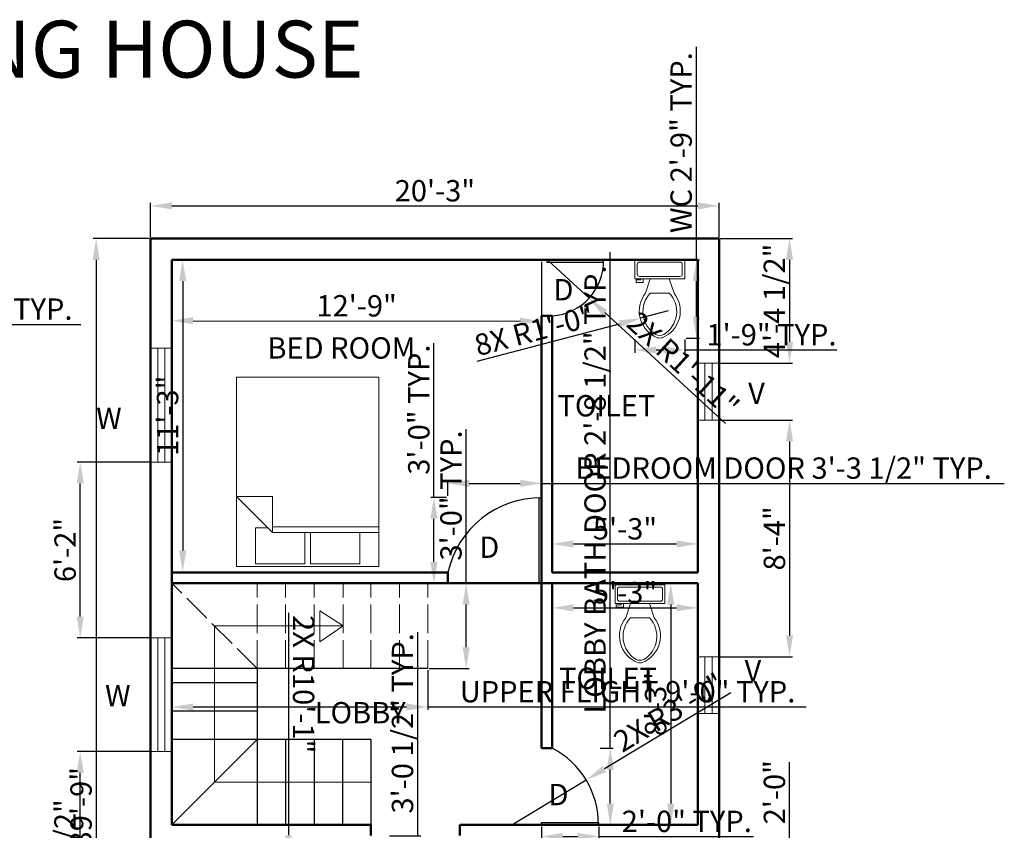
# Model space of a CAD drawing. Units: inches. Extents: x 1802 to 2621, y 1038 to 1686.
# Tile 5 of 5: x 2205 to 2621, y 1344 to 1686. Entities that reach past the tile are written whole.
import ezdxf

# ---------------------------------------------------------------- set-up
doc = ezdxf.new("R2010")
doc.units = ezdxf.units.IN
doc.linetypes.add('ACAD_ISO02W100', pattern=[15, 12, -3])
for name, color, linetype, lineweight in [('A-ANNO-DIMS', 2, 'Continuous', 18), ('A-ANNO-SYMB', 7, 'Continuous', 18), ('A-ANNO-TEXT', 7, 'Continuous', 18), ('A-AREA-IDEN', 7, 'Continuous', 25), ('A-DOOR', 3, 'Continuous', 25), ('A-FLOR-FIXT', 9, 'Continuous', 18), ('A-FLOR-STRS', 7, 'Continuous', 25), ('A-FLOR-STRS-OVHD', 8, 'ACAD_ISO02W100', 18), ('A-FURN', 8, 'Continuous', 18), ('A-GLAZ', 4, 'Continuous', 18), ('A-WALL', 7, 'Continuous', 50)]:
    doc.layers.add(name, color=color, linetype=linetype, lineweight=lineweight)
doc.styles.get("Standard").update_dxf_attribs({"font": 'arial.ttf'})
doc.dimstyles.new('ISO-25', dxfattribs={"dimtxt": 9, "dimasz": 9, "dimexe": 1.25, "dimexo": 0.625, "dimtad": 1, "dimdec": 1, "dimrnd": 9, "dimlunit": 3, "dimtxsty": 'Standard', "dimcen": 2.5, "dimadec": 0, "dimazin": 0, "dimtfac": 1, "dimtdec": 1, "dimtmove": 0, "dimatfit": 3, "dimfxl": 1, "dimarcsym": 0})

# ---------------------------------------------------------------- blocks, each defined once
blk = doc.blocks.new('*D20')
at = {"layer": 'A-ANNO-DIMS', "color": 0, "lineweight": -2, "transparency": 16777216}
for p, q in [((2269.56, 1583.93), (2269.52, 1557.61)), ((2425.56, 1583.74), (2425.52, 1557.42)), ((2278.53, 1558.85), (2416.53, 1558.68))]:
    blk.add_line(p, q, dxfattribs=at)
at = {"layer": 'A-ANNO-DIMS', "color": 0, "transparency": 16777216}
for points in [[(2278.53, 1560.35), (2278.52, 1557.35), (2269.53, 1558.86)], [(2416.53, 1560.18), (2416.52, 1557.18), (2425.53, 1558.67)]]:
    blk.add_solid(points, dxfattribs=at)
at = {"layer": 'Defpoints', "color": 0, "transparency": 16777216}
for p in [(2269.56, 1584.56), (2425.56, 1584.37), (2425.53, 1558.67)]:
    blk.add_point(p, dxfattribs=at)
at = {"layer": 'A-ANNO-DIMS', "color": 0, "transparency": 16777216, "insert": (2347.53, 1563.99), "char_height": 9, "attachment_point": 5, "rotation": 359.9308}
blk.add_mtext('12\'-9"', dxfattribs=at)
blk = doc.blocks.new('*D19')
at = {"layer": 'A-ANNO-DIMS', "color": 0, "lineweight": -2, "transparency": 16777216}
for p, q in [((2270.18, 1584.56), (2275.36, 1584.56)), ((2274.11, 1575.56), (2274.11, 1461.93)), ((2270.18, 1452.93), (2275.36, 1452.93))]:
    blk.add_line(p, q, dxfattribs=at)
at = {"layer": 'A-ANNO-DIMS', "color": 0, "transparency": 16777216}
for points in [[(2272.61, 1575.56), (2275.61, 1575.56), (2274.11, 1584.56)], [(2272.61, 1461.93), (2275.61, 1461.93), (2274.11, 1452.93)]]:
    blk.add_solid(points, dxfattribs=at)
at = {"layer": 'Defpoints', "color": 0, "transparency": 16777216}
for p in [(2269.56, 1584.56), (2269.56, 1452.93), (2274.11, 1452.93)]:
    blk.add_point(p, dxfattribs=at)
at = {"layer": 'A-ANNO-DIMS', "color": 0, "transparency": 16777216, "insert": (2268.89, 1518.75), "char_height": 9, "attachment_point": 5, "rotation": 90}
blk.add_mtext('11\'-3"', dxfattribs=at)
blk = doc.blocks.new('*D21')
at = {"layer": 'A-ANNO-DIMS', "color": 0, "lineweight": -2, "transparency": 16777216}
for p, q in [((2260.56, 1594.18), (2260.56, 1608.58)), ((2500.56, 1594.18), (2500.56, 1608.58)), ((2269.56, 1607.33), (2491.56, 1607.33))]:
    blk.add_line(p, q, dxfattribs=at)
at = {"layer": 'A-ANNO-DIMS', "color": 0, "transparency": 16777216}
for points in [[(2269.56, 1608.83), (2269.56, 1605.83), (2260.56, 1607.33)], [(2491.56, 1608.83), (2491.56, 1605.83), (2500.56, 1607.33)]]:
    blk.add_solid(points, dxfattribs=at)
at = {"layer": 'Defpoints', "color": 0, "transparency": 16777216}
for p in [(2500.56, 1607.33), (2260.56, 1593.56), (2500.56, 1593.56)]:
    blk.add_point(p, dxfattribs=at)
at = {"layer": 'A-ANNO-DIMS', "color": 0, "transparency": 16777216, "insert": (2380.56, 1612.56), "char_height": 9, "attachment_point": 5}
blk.add_mtext('20\'-3"', dxfattribs=at)
blk = doc.blocks.new('*D22')
at = {"layer": 'A-ANNO-DIMS', "color": 0, "lineweight": -2, "transparency": 16777216}
for p, q in [((2259.93, 1593.56), (2236.33, 1593.56)), ((2237.58, 1584.56), (2237.58, 1122.56)), ((2259.93, 1113.56), (2236.33, 1113.56))]:
    blk.add_line(p, q, dxfattribs=at)
at = {"layer": 'A-ANNO-DIMS', "color": 0, "transparency": 16777216}
for points in [[(2236.08, 1584.56), (2239.08, 1584.56), (2237.58, 1593.56)], [(2236.08, 1122.56), (2239.08, 1122.56), (2237.58, 1113.56)]]:
    blk.add_solid(points, dxfattribs=at)
at = {"layer": 'Defpoints', "color": 0, "transparency": 16777216}
for p in [(2260.56, 1593.56), (2237.58, 1113.56), (2260.56, 1113.56)]:
    blk.add_point(p, dxfattribs=at)
at = {"layer": 'A-ANNO-DIMS', "color": 0, "transparency": 16777216, "insert": (2232.36, 1353.56), "char_height": 9, "attachment_point": 5, "rotation": 90}
blk.add_mtext('39\'-9"', dxfattribs=at)
blk = doc.blocks.new('*D23')
at = {"layer": 'A-ANNO-DIMS', "color": 0, "lineweight": -2, "transparency": 16777216}
for p, q in [((2430.06, 1453.18), (2430.06, 1465.91)), ((2439.06, 1464.66), (2482.56, 1464.66)), ((2491.56, 1453.18), (2491.56, 1465.91))]:
    blk.add_line(p, q, dxfattribs=at)
at = {"layer": 'A-ANNO-DIMS', "color": 0, "transparency": 16777216}
for points in [[(2439.06, 1466.16), (2439.06, 1463.16), (2430.06, 1464.66)], [(2482.56, 1466.16), (2482.56, 1463.16), (2491.56, 1464.66)]]:
    blk.add_solid(points, dxfattribs=at)
at = {"layer": 'Defpoints', "color": 0, "transparency": 16777216}
for p in [(2491.56, 1464.66), (2430.06, 1452.56), (2491.56, 1452.56)]:
    blk.add_point(p, dxfattribs=at)
at = {"layer": 'A-ANNO-DIMS', "color": 0, "transparency": 16777216, "insert": (2460.81, 1469.88), "char_height": 9, "attachment_point": 5}
blk.add_mtext('5\'-3"', dxfattribs=at)
blk = doc.blocks.new('*D24')
at = {"layer": 'A-ANNO-DIMS', "color": 0, "lineweight": -2, "transparency": 16777216}
for p, q in [((2490.93, 1448.06), (2478.86, 1448.06)), ((2480.11, 1439.06), (2480.11, 1355.06)), ((2490.93, 1346.06), (2478.86, 1346.06))]:
    blk.add_line(p, q, dxfattribs=at)
at = {"layer": 'A-ANNO-DIMS', "color": 0, "transparency": 16777216}
for points in [[(2478.61, 1439.06), (2481.61, 1439.06), (2480.11, 1448.06)], [(2478.61, 1355.06), (2481.61, 1355.06), (2480.11, 1346.06)]]:
    blk.add_solid(points, dxfattribs=at)
at = {"layer": 'Defpoints', "color": 0, "transparency": 16777216}
for p in [(2491.56, 1448.06), (2480.11, 1346.06), (2491.56, 1346.06)]:
    blk.add_point(p, dxfattribs=at)
at = {"layer": 'A-ANNO-DIMS', "color": 0, "transparency": 16777216, "insert": (2474.89, 1397.06), "char_height": 9, "attachment_point": 5, "rotation": 90}
blk.add_mtext('8\'-3"', dxfattribs=at)
blk = doc.blocks.new('*D26')
at = {"layer": 'A-ANNO-DIMS', "color": 0, "lineweight": -2, "transparency": 16777216}
for p, q in [((2430.06, 1447.43), (2430.06, 1436.45)), ((2491.56, 1447.43), (2491.56, 1436.45)), ((2439.06, 1437.7), (2482.56, 1437.7))]:
    blk.add_line(p, q, dxfattribs=at)
at = {"layer": 'A-ANNO-DIMS', "color": 0, "transparency": 16777216}
for points in [[(2439.06, 1439.2), (2439.06, 1436.2), (2430.06, 1437.7)], [(2482.56, 1439.2), (2482.56, 1436.2), (2491.56, 1437.7)]]:
    blk.add_solid(points, dxfattribs=at)
at = {"layer": 'Defpoints', "color": 0, "transparency": 16777216}
for p in [(2430.06, 1448.06), (2491.56, 1448.06), (2491.56, 1437.7)]:
    blk.add_point(p, dxfattribs=at)
at = {"layer": 'A-ANNO-DIMS', "color": 0, "transparency": 16777216, "insert": (2460.81, 1442.92), "char_height": 9, "attachment_point": 5}
blk.add_mtext('5\'-3"', dxfattribs=at)
blk = doc.blocks.new('Bed - Queen')
for p, q in [((0, -80.00003), (0, 0)), ((0, 0), (59.99999, 0)), ((59.99999, 0), (59.99999, -80.00003)), ((7.99999, -1.2), (28.79998, -1.2)), ((7.99999, -14.4), (7.99999, -1.2)), ((28.79998, -1.2), (28.79998, -14.4)), ((31.19999, -1.2), (51.99999, -1.2)), ((31.19999, -14.4), (31.19999, -1.2)), ((51.99999, -1.2), (51.99999, -16.4)), ((0, -14.4), (44.8, -14.4)), ((59.99999, -29.6), (44.8, -14.4)), ((44.8, -14.4), (44.8, -29.6)), ((51.99999, -16.4), (46.79936, -16.4)), ((44.8, -16.8), (0, -16.8)), ((44.8, -29.6), (59.99999, -29.6)), ((59.99999, -80.00003), (0, -80.00003))]:
    blk.add_line(p, q)
blk = doc.blocks.new('Toilet - top')
for p, q in [((9.5, -6), (9.5, -2)), ((-8, -8.5), (-8, -8)), ((-7, -8), (-7, -9.5)), ((-4, -8), (-6, -14)), ((4, -8), (6, -14)), ((-10, -8.5), (-8, -8.5)), ((-10, -9.5), (-10, -8.5)), ((-7, -9.5), (-10, -9.5)), ((4, -14), (-4, -14))]:
    blk.add_line(p, q)
blk.add_lwpolyline([(10.5, -8), (10.5, 0), (-10.5, 0), (-10.5, -8)], close=True)
for points in [[(-9.5, -2), (-9.5, -6)], [(8.5, -1), (-8.5, -1)], [(-8.5, -7), (8.5, -7)]]:
    blk.add_lwpolyline(points)
for centre, radius, start, end in [((-8.62, -1.88), 0.884, 81.8699, 188.1301), ((8.62, -1.88), 0.884, 351.8699, 98.1301), ((-8.62, -6.12), 0.884, 171.8699, 278.1301), ((8.62, -6.12), 0.884, 261.8699, 8.1301), ((3.52, -21.58), 12.17, 141.4691, 247.9714), ((4.2, -21.82), 11.33, 136.3677, 238.9468), ((-3.52, -21.58), 12.17, 292.0284, 38.5307), ((-4.2, -21.82), 11.33, 301.053, 43.6321), ((0, -27.88), 4, 245.7318, 294.2682), ((0, -29), 4, 254.8605, 285.1395)]:
    blk.add_arc(centre, radius, start, end)
blk = doc.blocks.new('WIN-48IN')
for p, q in [((9, 48), (0, 48)), ((3, 48), (3, 0)), ((6, 48), (6, 0)), ((9, 0), (0, 0))]:
    blk.add_line(p, q)
blk = doc.blocks.new('VENT-24IN')
for p, q in [((0, 24), (9, 24)), ((3, 0), (3, 24)), ((6, 0), (6, 24)), ((0, 0), (9, 0))]:
    blk.add_line(p, q)
blk = doc.blocks.new('DOOR-BATH-REAR-24IN')
for p, q in [((0, 23.6), (0, 22.6)), ((0, 22.6), (24, 22.6)), ((24, 22.6), (24, 23.6))]:
    blk.add_line(p, q)
blk.add_arc((0.86, 23.1), 23.15, 273.6095, 1.2378)
blk = doc.blocks.new('DOOR-BEDROOM-36IN')
for p, q in [((38.47, 0), (38.47, 36)), ((38.47, 36), (39.47, 36)), ((39.47, 0), (38.47, 0))]:
    blk.add_line(p, q)
blk.add_arc((38.97, -3.86), 39.86, 89.2813, 167.8967)
blk = doc.blocks.new('DOOR-BATH-LOBBY-24IN')
for p, q in [((0, 0), (0, 1)), ((0, 1), (24, 1)), ((24, 1), (24, 0))]:
    blk.add_line(p, q)
blk.add_arc((-11.84, 0.5), 35.84, 359.2007, 62.8783)
blk = doc.blocks.new('STAIR-DIRECTION-U')
for p, q in [((44.37, 59.29), (44.37, 72.31)), ((44.37, 72.31), (54.34, 66)), ((0, 0), (0, 66)), ((0, 66), (54.34, 66)), ((54.34, 66), (44.37, 59.29)), ((66, 0), (0, 0))]:
    blk.add_line(p, q)
blk = doc.blocks.new('STAIR-WINDER-UPPER-TREADS')
for p, q in [((36, 0), (0, 36)), ((36, 0), (36, 36)), ((48, 0), (48, 36)), ((60, 0), (60, 36)), ((72.34, 0), (72.34, 36)), ((84, 0), (84, 36)), ((96, 0), (96, 36)), ((108, 0), (108, 36))]:
    blk.add_line(p, q)
blk = doc.blocks.new('STAIR-WINDER-VISIBLE')
for p, q in [((108, 66), (0, 66)), ((36, 66), (36, 0)), ((36, 60), (0, 60)), ((36, 48), (0, 48)), ((84, 36), (0, 36)), ((36, 36), (0, 0)), ((48, 36), (48, 0)), ((60, 36), (60, 0)), ((72, 36), (72, 0)), ((84, 36), (84, 0))]:
    blk.add_line(p, q)
blk = doc.blocks.new('*D41')
at = {"layer": 'A-ANNO-DIMS', "color": 0, "lineweight": -2, "transparency": 16777216}
for p, q in [((2490.95, 1584.56), (2490.95, 1674.48)), ((2486.61, 1584.56), (2492.2, 1584.56)), ((2490.95, 1560.51), (2490.95, 1575.56)), ((2486.61, 1551.51), (2492.2, 1551.51))]:
    blk.add_line(p, q, dxfattribs=at)
at = {"layer": 'A-ANNO-DIMS', "color": 0, "transparency": 16777216}
for points in [[(2489.45, 1575.56), (2492.45, 1575.56), (2490.95, 1584.56)], [(2489.45, 1560.51), (2492.45, 1560.51), (2490.95, 1551.51)]]:
    blk.add_solid(points, dxfattribs=at)
at = {"layer": 'Defpoints', "color": 0, "transparency": 16777216}
for p in [(2485.99, 1584.56), (2490.95, 1584.56), (2485.99, 1551.51)]:
    blk.add_point(p, dxfattribs=at)
at = {"layer": 'A-ANNO-DIMS', "color": 0, "transparency": 16777216, "insert": (2485.67, 1634.02), "char_height": 9, "attachment_point": 5, "rotation": 90}
blk.add_mtext('WC 2\'-9" TYP.', dxfattribs=at)
blk = doc.blocks.new('*D42')
at = {"layer": 'A-ANNO-DIMS', "color": 0, "lineweight": -2, "transparency": 16777216}
for p, q in [((2464.99, 1550.89), (2464.99, 1545.3)), ((2485.99, 1550.89), (2485.99, 1545.3)), ((2473.99, 1546.55), (2476.99, 1546.55)), ((2485.99, 1546.55), (2550.25, 1546.55))]:
    blk.add_line(p, q, dxfattribs=at)
at = {"layer": 'A-ANNO-DIMS', "color": 0, "transparency": 16777216}
for points in [[(2473.99, 1548.05), (2473.99, 1545.05), (2464.99, 1546.55)], [(2476.99, 1548.05), (2476.99, 1545.05), (2485.99, 1546.55)]]:
    blk.add_solid(points, dxfattribs=at)
at = {"layer": 'Defpoints', "color": 0, "transparency": 16777216}
for p in [(2464.99, 1551.51), (2485.99, 1551.51), (2485.99, 1546.55)]:
    blk.add_point(p, dxfattribs=at)
at = {"layer": 'A-ANNO-DIMS', "color": 0, "transparency": 16777216, "insert": (2522.62, 1551.77), "char_height": 9, "attachment_point": 5}
blk.add_mtext('1\'-9" TYP.', dxfattribs=at)
blk = doc.blocks.new('*D46')
at = {"layer": 'A-ANNO-DIMS', "color": 0, "lineweight": -2, "transparency": 16777216}
for p, q in [((2373.33, 1341.41), (2373.33, 1427.48)), ((2361.36, 1341.41), (2374.58, 1341.41)), ((2373.33, 1313.74), (2373.33, 1332.41)), ((2361.36, 1304.74), (2374.58, 1304.74))]:
    blk.add_line(p, q, dxfattribs=at)
at = {"layer": 'A-ANNO-DIMS', "color": 0, "transparency": 16777216}
for points in [[(2371.83, 1332.41), (2374.83, 1332.41), (2373.33, 1341.41)], [(2371.83, 1313.74), (2374.83, 1313.74), (2373.33, 1304.74)]]:
    blk.add_solid(points, dxfattribs=at)
at = {"layer": 'Defpoints', "color": 0, "transparency": 16777216}
for p in [(2360.73, 1341.41), (2373.33, 1341.41), (2360.73, 1304.74)]:
    blk.add_point(p, dxfattribs=at)
at = {"layer": 'A-ANNO-DIMS', "color": 0, "transparency": 16777216, "insert": (2368.05, 1388.94), "char_height": 9, "attachment_point": 5, "rotation": 90}
blk.add_mtext('3\'-0 1/2" TYP.', dxfattribs=at)
blk = doc.blocks.new('*D49')
at = {"layer": 'A-ANNO-DIMS', "color": 0, "lineweight": -2, "transparency": 16777216}
for p, q in [((2042.91, 1560.33), (2042.91, 1556.07)), ((2067.18, 1560.33), (2067.18, 1556.07)), ((2051.91, 1557.32), (2058.18, 1557.32)), ((2067.18, 1557.32), (2231.1, 1557.32))]:
    blk.add_line(p, q, dxfattribs=at)
at = {"layer": 'A-ANNO-DIMS', "color": 0, "transparency": 16777216}
for points in [[(2051.91, 1558.82), (2051.91, 1555.82), (2042.91, 1557.32)], [(2058.18, 1558.82), (2058.18, 1555.82), (2067.18, 1557.32)]]:
    blk.add_solid(points, dxfattribs=at)
at = {"layer": 'Defpoints', "color": 0, "transparency": 16777216}
for p in [(2042.91, 1560.96), (2067.18, 1560.96), (2067.18, 1557.32)]:
    blk.add_point(p, dxfattribs=at)
at = {"layer": 'A-ANNO-DIMS', "color": 0, "transparency": 16777216, "insert": (2153.64, 1562.6), "char_height": 9, "attachment_point": 5}
blk.add_mtext('BATH DOOR 2\'-0 1/2" TYP.', dxfattribs=at)
blk = doc.blocks.new('*D51')
at = {"layer": 'A-ANNO-DIMS', "color": 0, "lineweight": -2, "transparency": 16777216}
for p, q in [((2386.08, 1484.92), (2386.08, 1491.47)), ((2395.08, 1490.22), (2416.56, 1490.22)), ((2425.56, 1484.92), (2425.56, 1491.47)), ((2425.56, 1490.22), (2620.91, 1490.22))]:
    blk.add_line(p, q, dxfattribs=at)
at = {"layer": 'A-ANNO-DIMS', "color": 0, "transparency": 16777216}
for points in [[(2395.08, 1491.72), (2395.08, 1488.72), (2386.08, 1490.22)], [(2416.56, 1491.72), (2416.56, 1488.72), (2425.56, 1490.22)]]:
    blk.add_solid(points, dxfattribs=at)
at = {"layer": 'Defpoints', "color": 0, "transparency": 16777216}
for p in [(2425.56, 1490.22), (2386.08, 1484.3), (2425.56, 1484.3)]:
    blk.add_point(p, dxfattribs=at)
at = {"layer": 'A-ANNO-DIMS', "color": 0, "transparency": 16777216, "insert": (2527.73, 1495.5), "char_height": 9, "attachment_point": 5}
blk.add_mtext('BEDROOM DOOR 3\'-3 1/2" TYP.', dxfattribs=at)
blk = doc.blocks.new('*D52')
at = {"layer": 'A-ANNO-DIMS', "color": 0, "lineweight": -2, "transparency": 16777216}
for p, q in [((2380.16, 1484.3), (2380.16, 1549.4)), ((2385.46, 1484.3), (2378.91, 1484.3)), ((2380.16, 1457.06), (2380.16, 1475.3)), ((2385.46, 1448.06), (2378.91, 1448.06))]:
    blk.add_line(p, q, dxfattribs=at)
at = {"layer": 'A-ANNO-DIMS', "color": 0, "transparency": 16777216}
for points in [[(2378.66, 1475.3), (2381.66, 1475.3), (2380.16, 1484.3)], [(2378.66, 1457.06), (2381.66, 1457.06), (2380.16, 1448.06)]]:
    blk.add_solid(points, dxfattribs=at)
at = {"layer": 'Defpoints', "color": 0, "transparency": 16777216}
for p in [(2380.16, 1484.3), (2386.08, 1484.3), (2386.08, 1448.06)]:
    blk.add_point(p, dxfattribs=at)
at = {"layer": 'A-ANNO-DIMS', "color": 0, "transparency": 16777216, "insert": (2374.94, 1521.35), "char_height": 9, "attachment_point": 5, "rotation": 90}
blk.add_mtext('3\'-0" TYP.', dxfattribs=at)
blk = doc.blocks.new('*D53')
at = {"layer": 'A-ANNO-DIMS', "color": 0, "lineweight": -2, "transparency": 16777216}
for p, q in [((2454.61, 1378.46), (2454.61, 1587.8)), ((2450.37, 1378.46), (2455.86, 1378.46)), ((2454.61, 1355.06), (2454.61, 1369.46)), ((2450.37, 1346.06), (2455.86, 1346.06))]:
    blk.add_line(p, q, dxfattribs=at)
at = {"layer": 'A-ANNO-DIMS', "color": 0, "transparency": 16777216}
for points in [[(2453.11, 1369.46), (2456.11, 1369.46), (2454.61, 1378.46)], [(2453.11, 1355.06), (2456.11, 1355.06), (2454.61, 1346.06)]]:
    blk.add_solid(points, dxfattribs=at)
at = {"layer": 'Defpoints', "color": 0, "transparency": 16777216}
for p in [(2449.75, 1378.46), (2454.61, 1378.46), (2449.75, 1346.06)]:
    blk.add_point(p, dxfattribs=at)
at = {"layer": 'A-ANNO-DIMS', "color": 0, "transparency": 16777216, "insert": (2449.33, 1487.63), "char_height": 9, "attachment_point": 5, "rotation": 90}
blk.add_mtext('LOBBY BATH DOOR 2\'-8 1/2" TYP.', dxfattribs=at)
blk = doc.blocks.new('*D54')
at = {"layer": 'A-ANNO-DIMS', "color": 0, "lineweight": -2, "transparency": 16777216}
for p, q in [((2425.56, 1345.43), (2425.56, 1339.95)), ((2449.75, 1345.43), (2449.75, 1339.95)), ((2434.56, 1341.2), (2440.75, 1341.2)), ((2449.75, 1341.2), (2515.01, 1341.2))]:
    blk.add_line(p, q, dxfattribs=at)
at = {"layer": 'A-ANNO-DIMS', "color": 0, "transparency": 16777216}
for points in [[(2434.56, 1342.7), (2434.56, 1339.7), (2425.56, 1341.2)], [(2440.75, 1342.7), (2440.75, 1339.7), (2449.75, 1341.2)]]:
    blk.add_solid(points, dxfattribs=at)
at = {"layer": 'Defpoints', "color": 0, "transparency": 16777216}
for p in [(2425.56, 1346.06), (2449.75, 1346.06), (2449.75, 1341.2)]:
    blk.add_point(p, dxfattribs=at)
at = {"layer": 'A-ANNO-DIMS', "color": 0, "transparency": 16777216, "insert": (2486.88, 1346.42), "char_height": 9, "attachment_point": 5}
blk.add_mtext('2\'-0" TYP.', dxfattribs=at)
blk = doc.blocks.new('*D57')
at = {"layer": 'A-ANNO-DIMS', "color": 0, "lineweight": -2, "transparency": 16777216}
for p, q in [((2269.56, 1411.43), (2269.56, 1394.61)), ((2377.56, 1411.43), (2377.56, 1394.61)), ((2278.56, 1395.86), (2368.56, 1395.86)), ((2377.56, 1395.86), (2537.21, 1395.86))]:
    blk.add_line(p, q, dxfattribs=at)
at = {"layer": 'A-ANNO-DIMS', "color": 0, "transparency": 16777216}
for points in [[(2278.56, 1397.36), (2278.56, 1394.36), (2269.56, 1395.86)], [(2368.56, 1397.36), (2368.56, 1394.36), (2377.56, 1395.86)]]:
    blk.add_solid(points, dxfattribs=at)
at = {"layer": 'Defpoints', "color": 0, "transparency": 16777216}
for p in [(2269.56, 1412.06), (2377.56, 1412.06), (2377.56, 1395.86)]:
    blk.add_point(p, dxfattribs=at)
at = {"layer": 'A-ANNO-DIMS', "color": 0, "transparency": 16777216, "insert": (2461.88, 1401.14), "char_height": 9, "attachment_point": 5}
blk.add_mtext('UPPER FLIGHT 9\'-0" TYP.', dxfattribs=at)
blk = doc.blocks.new('*D58')
at = {"layer": 'A-ANNO-DIMS', "color": 0, "lineweight": -2, "transparency": 16777216}
for p, q in [((2393.76, 1448.06), (2393.76, 1513.16)), ((2378.18, 1448.06), (2395.01, 1448.06)), ((2393.76, 1421.06), (2393.76, 1439.06)), ((2378.18, 1412.06), (2395.01, 1412.06))]:
    blk.add_line(p, q, dxfattribs=at)
at = {"layer": 'A-ANNO-DIMS', "color": 0, "transparency": 16777216}
for points in [[(2392.26, 1439.06), (2395.26, 1439.06), (2393.76, 1448.06)], [(2392.26, 1421.06), (2395.26, 1421.06), (2393.76, 1412.06)]]:
    blk.add_solid(points, dxfattribs=at)
at = {"layer": 'Defpoints', "color": 0, "transparency": 16777216}
for p in [(2377.56, 1448.06), (2393.76, 1448.06), (2377.56, 1412.06)]:
    blk.add_point(p, dxfattribs=at)
at = {"layer": 'A-ANNO-DIMS', "color": 0, "transparency": 16777216, "insert": (2388.53, 1485.11), "char_height": 9, "attachment_point": 5, "rotation": 90}
blk.add_mtext('3\'-0" TYP.', dxfattribs=at)
blk = doc.blocks.new('*D68')
at = {"layer": 'A-ANNO-DIMS', "color": 0, "lineweight": -2, "transparency": 16777216}
for p, q in [((2259.93, 1377), (2229.61, 1377)), ((2230.86, 1297.57), (2230.86, 1368)), ((2259.93, 1288.57), (2229.61, 1288.57))]:
    blk.add_line(p, q, dxfattribs=at)
at = {"layer": 'A-ANNO-DIMS', "color": 0, "transparency": 16777216}
for points in [[(2229.36, 1368), (2232.36, 1368), (2230.86, 1377)], [(2229.36, 1297.57), (2232.36, 1297.57), (2230.86, 1288.57)]]:
    blk.add_solid(points, dxfattribs=at)
at = {"layer": 'Defpoints', "color": 0, "transparency": 16777216}
for p in [(2230.86, 1377), (2260.56, 1377), (2260.56, 1288.57)]:
    blk.add_point(p, dxfattribs=at)
at = {"layer": 'A-ANNO-DIMS', "color": 0, "transparency": 16777216, "insert": (2225.58, 1332.78), "char_height": 9, "attachment_point": 5, "rotation": 90}
blk.add_mtext('7\'-4 1/2"', dxfattribs=at)
blk = doc.blocks.new('*D69')
at = {"layer": 'A-ANNO-DIMS', "color": 0, "lineweight": -2, "transparency": 16777216}
for p, q in [((2259.93, 1499.22), (2229.61, 1499.22)), ((2230.86, 1434), (2230.86, 1490.22)), ((2259.93, 1425), (2229.61, 1425))]:
    blk.add_line(p, q, dxfattribs=at)
at = {"layer": 'A-ANNO-DIMS', "color": 0, "transparency": 16777216}
for points in [[(2229.36, 1490.22), (2232.36, 1490.22), (2230.86, 1499.22)], [(2229.36, 1434), (2232.36, 1434), (2230.86, 1425)]]:
    blk.add_solid(points, dxfattribs=at)
at = {"layer": 'Defpoints', "color": 0, "transparency": 16777216}
for p in [(2230.86, 1499.22), (2260.56, 1499.22), (2260.56, 1425)]:
    blk.add_point(p, dxfattribs=at)
at = {"layer": 'A-ANNO-DIMS', "color": 0, "transparency": 16777216, "insert": (2225.64, 1462.11), "char_height": 9, "attachment_point": 5, "rotation": 90}
blk.add_mtext('6\'-2"', dxfattribs=at)
blk = doc.blocks.new('*D70')
at = {"layer": 'A-ANNO-DIMS', "color": 0, "lineweight": -2, "transparency": 16777216}
for p, q in [((2501.18, 1593.56), (2531.51, 1593.56)), ((2530.26, 1584.56), (2530.26, 1549.93)), ((2501.18, 1540.93), (2531.51, 1540.93))]:
    blk.add_line(p, q, dxfattribs=at)
at = {"layer": 'A-ANNO-DIMS', "color": 0, "transparency": 16777216}
for points in [[(2528.76, 1584.56), (2531.76, 1584.56), (2530.26, 1593.56)], [(2528.76, 1549.93), (2531.76, 1549.93), (2530.26, 1540.93)]]:
    blk.add_solid(points, dxfattribs=at)
at = {"layer": 'Defpoints', "color": 0, "transparency": 16777216}
for p in [(2500.56, 1593.56), (2500.56, 1540.93), (2530.26, 1540.93)]:
    blk.add_point(p, dxfattribs=at)
at = {"layer": 'A-ANNO-DIMS', "color": 0, "transparency": 16777216, "insert": (2524.98, 1567.25), "char_height": 9, "attachment_point": 5, "rotation": 90}
blk.add_mtext('4\'-4 1/2"', dxfattribs=at)
blk = doc.blocks.new('*D71')
at = {"layer": 'A-ANNO-DIMS', "color": 0, "lineweight": -2, "transparency": 16777216}
for p, q in [((2501.18, 1516.93), (2531.51, 1516.93)), ((2530.26, 1507.93), (2530.26, 1426.08)), ((2501.18, 1417.08), (2531.51, 1417.08))]:
    blk.add_line(p, q, dxfattribs=at)
at = {"layer": 'A-ANNO-DIMS', "color": 0, "transparency": 16777216}
for points in [[(2528.76, 1507.93), (2531.76, 1507.93), (2530.26, 1516.93)], [(2528.76, 1426.08), (2531.76, 1426.08), (2530.26, 1417.08)]]:
    blk.add_solid(points, dxfattribs=at)
at = {"layer": 'Defpoints', "color": 0, "transparency": 16777216}
for p in [(2500.56, 1516.93), (2500.56, 1417.08), (2530.26, 1417.08)]:
    blk.add_point(p, dxfattribs=at)
at = {"layer": 'A-ANNO-DIMS', "color": 0, "transparency": 16777216, "insert": (2525.04, 1467.01), "char_height": 9, "attachment_point": 5, "rotation": 90}
blk.add_mtext('8\'-4"', dxfattribs=at)
blk = doc.blocks.new('*D76')
at = {"layer": 'A-ANNO-DIMS', "color": 0, "lineweight": -2, "transparency": 16777216}
for p, q in [((2530.26, 1338.22), (2530.26, 1372.54)), ((2391.68, 1338.22), (2531.51, 1338.22)), ((2530.26, 1323.41), (2530.26, 1329.22)), ((2391.68, 1314.41), (2531.51, 1314.41))]:
    blk.add_line(p, q, dxfattribs=at)
at = {"layer": 'A-ANNO-DIMS', "color": 0, "transparency": 16777216}
for points in [[(2528.76, 1329.22), (2531.76, 1329.22), (2530.26, 1338.22)], [(2528.76, 1323.41), (2531.76, 1323.41), (2530.26, 1314.41)]]:
    blk.add_solid(points, dxfattribs=at)
at = {"layer": 'Defpoints', "color": 0, "transparency": 16777216}
for p in [(2391.06, 1338.22), (2530.26, 1338.22), (2391.06, 1314.41)]:
    blk.add_point(p, dxfattribs=at)
at = {"layer": 'A-ANNO-DIMS', "color": 0, "transparency": 16777216, "insert": (2525.04, 1359.88), "char_height": 9, "attachment_point": 5, "rotation": 90}
blk.add_mtext('2\'-0"', dxfattribs=at)
blk = doc.blocks.new('*D82')
at = {"layer": 'A-ANNO-DIMS', "color": 0, "lineweight": -2, "transparency": 16777216}
for p, q in [((2505.5, 1401.79), (2452.14, 1369.68)), ((2413.72, 1346.56), (2444.43, 1365.04))]:
    blk.add_line(p, q, dxfattribs=at)
at = {"layer": 'A-ANNO-DIMS', "color": 0, "transparency": 16777216}
blk.add_solid([(2451.37, 1370.97), (2452.91, 1368.4), (2444.43, 1365.04)], dxfattribs=at)
at = {"layer": 'Defpoints', "color": 0, "transparency": 16777216}
for p in [(2444.43, 1365.04), (2413.72, 1346.56)]:
    blk.add_point(p, dxfattribs=at)
at = {"layer": 'A-ANNO-DIMS', "color": 0, "transparency": 16777216, "insert": (2479.98, 1392.53), "char_height": 9, "attachment_point": 5, "rotation": 31.0392}
blk.add_mtext('2X R3\'-0"', dxfattribs=at)
blk = doc.blocks.new('*D83')
at = {"layer": 'A-ANNO-DIMS', "color": 0, "lineweight": -2, "transparency": 16777216}
for p, q in [((2428.6, 1584.06), (2445.64, 1568.4)), ((2503.28, 1515.44), (2452.27, 1562.31))]:
    blk.add_line(p, q, dxfattribs=at)
at = {"layer": 'A-ANNO-DIMS', "color": 0, "transparency": 16777216}
blk.add_solid([(2453.29, 1563.41), (2451.26, 1561.2), (2445.64, 1568.4)], dxfattribs=at)
at = {"layer": 'Defpoints', "color": 0, "transparency": 16777216}
for p in [(2428.6, 1584.06), (2445.64, 1568.4)]:
    blk.add_point(p, dxfattribs=at)
at = {"layer": 'A-ANNO-DIMS', "color": 0, "transparency": 16777216, "insert": (2484.57, 1539.62), "char_height": 9, "attachment_point": 5, "rotation": 317.4234}
blk.add_mtext('2X R1\'-11"', dxfattribs=at)
blk = doc.blocks.new('*D84')
at = {"layer": 'A-ANNO-DIMS', "color": 0, "lineweight": -2, "transparency": 16777216}
for p, q in [((2318.73, 1435.59), (2318.73, 1341.74)), ((2318.73, 1211.54), (2318.73, 1332.74))]:
    blk.add_line(p, q, dxfattribs=at)
at = {"layer": 'A-ANNO-DIMS', "color": 0, "transparency": 16777216}
blk.add_solid([(2320.23, 1341.74), (2317.23, 1341.74), (2318.73, 1332.74)], dxfattribs=at)
at = {"layer": 'Defpoints', "color": 0, "transparency": 16777216}
for p in [(2318.73, 1332.74), (2318.73, 1211.54)]:
    blk.add_point(p, dxfattribs=at)
at = {"layer": 'A-ANNO-DIMS', "color": 0, "transparency": 16777216, "insert": (2323.95, 1405.46), "char_height": 9, "attachment_point": 5, "rotation": 270.0001}
blk.add_mtext('2X R10\'-1"', dxfattribs=at)
blk = doc.blocks.new('*D86')
at = {"layer": 'A-ANNO-DIMS', "color": 0, "lineweight": -2, "transparency": 16777216}
for p, q in [((2479.01, 1562.98), (2467.24, 1559.88)), ((2398.44, 1541.81), (2458.53, 1557.6))]:
    blk.add_line(p, q, dxfattribs=at)
at = {"layer": 'A-ANNO-DIMS', "color": 0, "transparency": 16777216}
blk.add_solid([(2458.15, 1559.05), (2458.92, 1556.15), (2467.24, 1559.88)], dxfattribs=at)
at = {"layer": 'Defpoints', "color": 0, "transparency": 16777216}
for p in [(2479.01, 1562.98), (2467.24, 1559.88)]:
    blk.add_point(p, dxfattribs=at)
at = {"layer": 'A-ANNO-DIMS', "color": 0, "transparency": 16777216, "insert": (2422.81, 1553.61), "char_height": 9, "attachment_point": 5, "rotation": 14.7201}
blk.add_mtext('8X R1\'-0"', dxfattribs=at)

msp = doc.modelspace()

# ---------------------------------------------------------------- linework, layer by layer
at = {"layer": 'A-WALL'}
for p, q in [((2500.56, 1593.56), (2260.56, 1593.56)), ((2260.56, 1593.56), (2260.56, 1113.56)), ((2500.56, 1113.56), (2500.56, 1593.56)), ((2491.56, 1584.56), (2269.56, 1584.56)), ((2269.56, 1584.56), (2269.56, 1346.06)), ((2491.56, 1452.56), (2491.56, 1584.56)), ((2425.56, 1560.96), (2425.56, 1378.46)), ((2425.56, 1560.96), (2430.06, 1560.96)), ((2430.06, 1560.96), (2430.06, 1452.56)), ((2386.08, 1452.56), (2269.56, 1452.56)), ((2386.08, 1452.56), (2386.08, 1448.06)), ((2491.56, 1452.56), (2430.06, 1452.56)), ((2491.56, 1448.06), (2269.56, 1448.06)), ((2430.06, 1448.06), (2430.06, 1378.46)), ((2491.56, 1346.06), (2491.56, 1448.06)), ((2430.06, 1378.46), (2425.56, 1378.46)), ((2353.56, 1346.06), (2269.56, 1346.06)), ((2353.56, 1346.06), (2353.56, 1341.56)), ((2425.56, 1346.06), (2391.06, 1346.06)), ((2391.06, 1341.56), (2391.06, 1346.06)), ((2491.56, 1346.06), (2425.56, 1346.06))]:
    msp.add_line(p, q, dxfattribs=at)

# ---------------------------------------------------------------- block references
at = {"layer": 'A-ANNO-SYMB'}
msp.add_blockref('STAIR-DIRECTION-U', (2287.56, 1364.06), dxfattribs=at)
at = {"layer": 'A-DOOR'}
for name, p in [('DOOR-BATH-REAR-24IN', (2427.74, 1560.96)), ('DOOR-BEDROOM-36IN', (2386.08, 1448.06)), ('DOOR-BATH-LOBBY-24IN', (2425.56, 1346.06))]:
    msp.add_blockref(name, p, dxfattribs=at)
at = {"layer": 'A-FLOR-FIXT'}
for p in [(2475.49, 1584.56), (2467.12, 1447.47)]:
    msp.add_blockref('Toilet - top', p, dxfattribs=at)
at = {"layer": 'A-FLOR-STRS'}
msp.add_blockref('STAIR-WINDER-VISIBLE', (2269.56, 1346.06), dxfattribs=at)
at = {"layer": 'A-FLOR-STRS-OVHD'}
msp.add_blockref('STAIR-WINDER-UPPER-TREADS', (2269.56, 1412.06), dxfattribs=at)
at = {"layer": 'A-FURN', "rotation": 180}
msp.add_blockref('Bed - Queen', (2356.87, 1455.09), dxfattribs=at)
at = {"layer": 'A-GLAZ', "rotation": 180}
for name, p in [('WIN-48IN', (2269.56, 1547.22)), ('VENT-24IN', (2500.56, 1540.93)), ('WIN-48IN', (2269.56, 1425)), ('VENT-24IN', (2500.56, 1417.08))]:
    msp.add_blockref(name, p, dxfattribs=at)

# ---------------------------------------------------------------- texts
at = {"layer": 'A-ANNO-TEXT', "attachment_point": 1}
for s, width, insert, char_height in [('SOUTH FACING HOUSE', 491.7378, (1999.67, 1685.48), 24), ('D ', 17.1074, (2430.62, 1576.43), 9), ('V', 21.5258, (2512.76, 1532.78), 9), ('W', 30.0361, (2237.58, 1522.22), 9), ('D ', 17.1074, (2399.3, 1467.77), 9), ('V', 21.5258, (2511.26, 1415.74), 9), ('W', 30.0361, (2241.33, 1405.18), 9), ('D ', 17.1074, (2428.53, 1363.38), 9)]:
    msp.add_mtext_dynamic_manual_height_columns(s, width=width, gutter_width=12.5, heights=[0], dxfattribs=dict(at, insert=insert, char_height=char_height))
at = {"layer": 'A-AREA-IDEN', "char_height": 9, "attachment_point": 1}
for s, insert in [('BED ROOM', (2309.84, 1551.87)), ('TOILET', (2432.31, 1527.48)), ('TOILET', (2432.94, 1412.44)), ('LOBBY', (2329.84, 1397.94))]:
    msp.add_mtext_dynamic_manual_height_columns(s, width=82.6611, gutter_width=12.5, heights=[0], dxfattribs=dict(at, insert=insert))

# ---------------------------------------------------------------- dimensions: what is measured, and where the dimension line sits
at = {"layer": 'A-ANNO-DIMS'}
for base, p1, p2, text, picture, middle in [((2490.9459, 1584.5576), (2485.989, 1551.5113), (2485.989, 1584.5576), 'WC <> TYP.', '*D41', (2485.6675, 1634.0165)), ((2454.61, 1378.46), (2449.75, 1346.06), (2449.75, 1378.46), 'LOBBY BATH DOOR <> TYP.', '*D53', (2449.33, 1487.63)), ((2380.16, 1484.3), (2386.08, 1448.06), (2386.08, 1484.3), '<> TYP.', '*D52', (2374.94, 1521.35)), ((2393.76, 1448.06), (2377.56, 1412.06), (2377.56, 1448.06), '<> TYP.', '*D58', (2388.53, 1485.11)), ((2373.33, 1341.41), (2360.73, 1304.74), (2360.73, 1341.41), '<> TYP.', '*D46', (2368.05, 1388.94))]:
    dim = msp.add_linear_dim(base=base, p1=p1, p2=p2, angle=90, text=text, dimstyle='ISO-25', override={"dimdec": 1, "dimlfac": 1, "dimrnd": 0, "dimzin": 1, "dimdsep": 46, "dimlunit": 4, "dimfrac": 2}, dxfattribs=at)
    dim.commit()
    dim.dimension.update_dxf_attribs({"geometry": picture, "text_midpoint": middle})
for base, p1, p2, picture, middle in [((2500.56, 1607.33), (2260.56, 1593.56), (2500.56, 1593.56), '*D21', (2380.56, 1612.56)), ((2491.56, 1464.66), (2430.06, 1452.56), (2491.56, 1452.56), '*D23', (2460.81, 1469.88)), ((2491.56, 1437.7), (2430.06, 1448.06), (2491.56, 1448.06), '*D26', (2460.81, 1442.92))]:
    dim = msp.add_linear_dim(base=base, p1=p1, p2=p2, dimstyle='ISO-25', override={"dimclrd": 0, "dimclre": 0, "dimclrt": 0}, dxfattribs=at)
    dim.commit()
    dim.dimension.update_dxf_attribs({"geometry": picture, "text_midpoint": middle})
for base, p1, p2, text, picture, middle in [((2067.18, 1557.32), (2042.91, 1560.96), (2067.18, 1560.96), 'BATH DOOR <> TYP.', '*D49', (2153.64, 1562.6)), ((2485.99, 1546.55), (2464.99, 1551.51), (2485.99, 1551.51), '<> TYP.', '*D42', (2522.62, 1551.77)), ((2425.56, 1490.22), (2386.08, 1484.3), (2425.56, 1484.3), 'BEDROOM DOOR <> TYP.', '*D51', (2527.73, 1495.5)), ((2377.56, 1395.86), (2269.56, 1412.06), (2377.56, 1412.06), 'UPPER FLIGHT <> TYP.', '*D57', (2461.88, 1401.14)), ((2449.75, 1341.2), (2425.56, 1346.06), (2449.75, 1346.06), '<> TYP.', '*D54', (2486.88, 1346.42))]:
    dim = msp.add_linear_dim(base=base, p1=p1, p2=p2, text=text, dimstyle='ISO-25', override={"dimdec": 1, "dimlfac": 1, "dimrnd": 0, "dimzin": 1, "dimdsep": 46, "dimlunit": 4, "dimfrac": 2}, dxfattribs=at)
    dim.commit()
    dim.dimension.update_dxf_attribs({"geometry": picture, "text_midpoint": middle})
for base, p1, p2, override, picture, middle in [((2237.58, 1113.56), (2260.56, 1593.56), (2260.56, 1113.56), {"dimclrd": 0, "dimclre": 0, "dimclrt": 0}, '*D22', (2232.36, 1353.56)), ((2530.26, 1540.93), (2500.56, 1593.56), (2500.56, 1540.93), {"dimdec": 1, "dimlfac": 1, "dimrnd": 0, "dimzin": 1, "dimdsep": 46, "dimlunit": 4, "dimfrac": 2}, '*D70', (2524.98, 1567.25)), ((2274.11, 1452.93), (2269.56, 1584.56), (2269.56, 1452.93), {"dimclrd": 0, "dimclre": 0, "dimclrt": 0}, '*D19', (2268.89, 1518.75)), ((2530.2565, 1417.0788), (2500.5565, 1516.935), (2500.5565, 1417.0788), {"dimdec": 1, "dimlfac": 1, "dimrnd": 0, "dimzin": 1, "dimdsep": 46, "dimlunit": 4, "dimfrac": 2}, '*D71', (2525.0364, 1467.0069)), ((2230.86, 1499.22), (2260.56, 1425), (2260.56, 1499.22), {"dimdec": 1, "dimlfac": 1, "dimrnd": 0, "dimzin": 1, "dimdsep": 46, "dimlunit": 4, "dimfrac": 2}, '*D69', (2225.64, 1462.11)), ((2480.11, 1346.06), (2491.56, 1448.06), (2491.56, 1346.06), {"dimclrd": 0, "dimclre": 0, "dimclrt": 0}, '*D24', (2474.89, 1397.06)), ((2230.86, 1377), (2260.56, 1288.57), (2260.56, 1377), {"dimdec": 1, "dimlfac": 1, "dimrnd": 0, "dimzin": 1, "dimdsep": 46, "dimlunit": 4, "dimfrac": 2}, '*D68', (2225.58, 1332.78)), ((2530.26, 1338.22), (2391.06, 1314.41), (2391.06, 1338.22), {"dimdec": 1, "dimlfac": 1, "dimrnd": 0, "dimzin": 1, "dimdsep": 46, "dimlunit": 4, "dimfrac": 2}, '*D76', (2525.04, 1359.88))]:
    dim = msp.add_linear_dim(base=base, p1=p1, p2=p2, angle=90, dimstyle='ISO-25', override=override, dxfattribs=at)
    dim.commit()
    dim.dimension.update_dxf_attribs({"geometry": picture, "text_midpoint": middle})
dim = msp.add_aligned_dim(p1=(2269.56, 1584.56), p2=(2425.56, 1584.37), distance=-25.7, dimstyle='ISO-25', override={"dimclrd": 0, "dimclre": 0, "dimclrt": 0}, dxfattribs=at)
dim.commit()
dim.dimension.update_dxf_attribs({"geometry": '*D20', "text_midpoint": (2347.53, 1563.99)})
for center, mpoint, text, picture, middle in [((2428.6, 1584.06), (2445.64, 1568.4), '2X <>', '*D83', (2484.57, 1539.62)), ((2479.01, 1562.98), (2467.24, 1559.88), '8X <>', '*D86', (2422.81, 1553.61)), ((2413.72, 1346.56), (2444.43, 1365.04), '2X <>', '*D82', (2479.98, 1392.53))]:
    dim = msp.add_radius_dim(center=center, mpoint=mpoint, text=text, dimstyle='ISO-25', override={"dimdec": 1, "dimlfac": 1, "dimrnd": 0, "dimzin": 1, "dimdsep": 46, "dimlunit": 4, "dimfrac": 2}, dxfattribs=at)
    dim.commit()
    dim.dimension.update_dxf_attribs({"geometry": picture, "text_midpoint": middle})
dim = msp.add_radius_dim(center=(2318.73, 1211.54), mpoint=(2318.73, 1332.74), text='2X <>', dimstyle='ISO-25', override={"dimdec": 1, "dimlfac": 1, "dimrnd": 0, "dimzin": 1, "dimdsep": 46, "dimlunit": 4, "dimfrac": 2}, dxfattribs=at)
dim.commit()
dim.dimension.update_dxf_attribs({"geometry": '*D84', "text_midpoint": (2318.73, 1405.46), "dimtype": 164})

doc.saveas('drawing.dxf')
